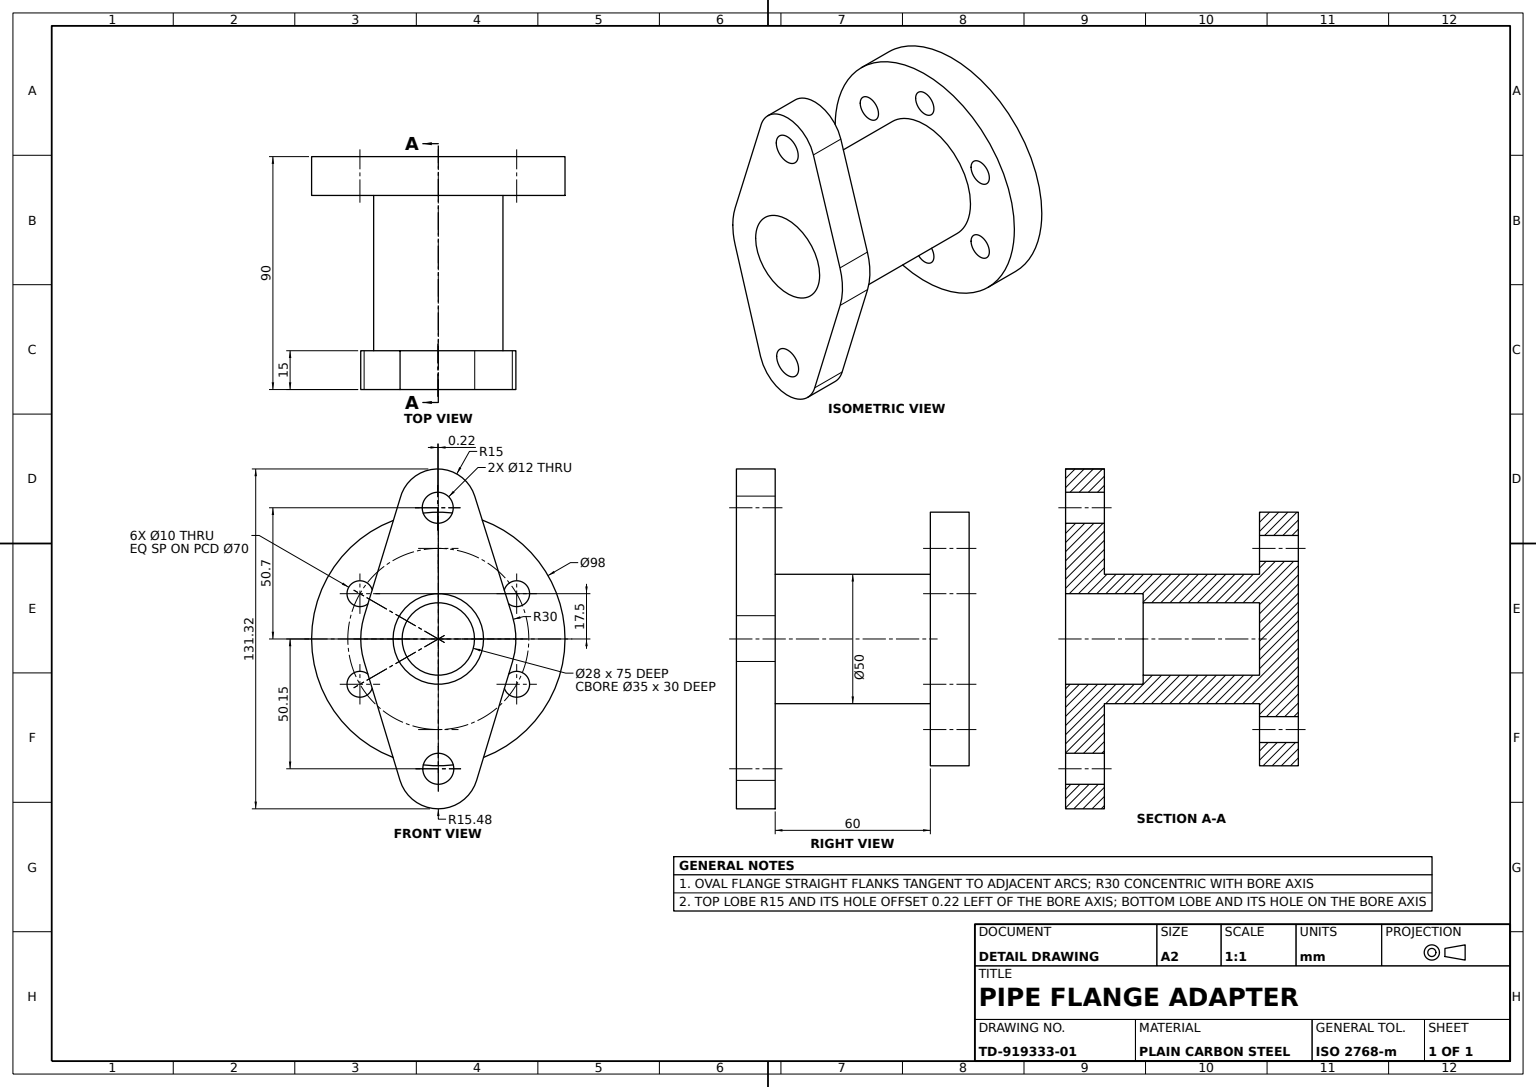
from build123d import *

# Parameters (mm, degrees)
ROUND_FLANGE_SKETCH_R          = 49
ROUND_FLANGE_98_DEPTH          = 15
ROUND_FLANGE_HOLES_SKETCH_R    = 5
ROUND_FLANGE_HOLES_6X_10_DEPTH = 15
SLEEVE_SKETCH_R                = 25
SLEEVE_50_DEPTH                = 60
OVAL_FLANGE_DEPTH              = 15
OVAL_FLANGE_HOLES_SKETCH_R     = 6
OVAL_FLANGE_HOLES_2X_12_DEPTH  = 15
COUNTERBORE_SKETCH_R           = 17.5
COUNTERBORE_35_DEPTH           = 30
BORE_SKETCH_R                  = 14
BORE_28_DEPTH                  = 45


with BuildPart() as part:
    # Round Flange Sketch → Round Flange Ø98 (new body)
    with BuildSketch(Plane.XY):
        Circle(ROUND_FLANGE_SKETCH_R)
    extrude(amount=ROUND_FLANGE_98_DEPTH)

    # Round Flange Holes Sketch → Round Flange Holes 6xØ10 (cut)
    with BuildSketch(Plane.XY.offset(15)):
        with Locations((0, 35)):
            Circle(ROUND_FLANGE_HOLES_SKETCH_R)
        with Locations((30.310889132, 17.5)):
            Circle(ROUND_FLANGE_HOLES_SKETCH_R)
        with Locations((30.310889132, -17.5)):
            Circle(ROUND_FLANGE_HOLES_SKETCH_R)
        with Locations((0, -35)):
            Circle(ROUND_FLANGE_HOLES_SKETCH_R)
        with Locations((-30.310889132, -17.5)):
            Circle(ROUND_FLANGE_HOLES_SKETCH_R)
        with Locations((-30.310889132, 17.5)):
            Circle(ROUND_FLANGE_HOLES_SKETCH_R)
    extrude(amount=-ROUND_FLANGE_HOLES_6X_10_DEPTH, mode=Mode.SUBTRACT)

    # Sleeve Sketch → Sleeve Ø50 (add)
    with BuildSketch(Plane.XY.offset(15)):
        Circle(SLEEVE_SKETCH_R)
    extrude(amount=SLEEVE_50_DEPTH)

    # Oval Flange Sketch → Oval Flange (add)
    with BuildSketch(Plane.XY.offset(75)):
        with BuildLine():
            Line((-14.812486777, -54.633777367), (-28.714375061, -8.688191115))
            ThreePointArc((-28.714375061, -8.688191115), (-29.999971167, 0.041592963), (-28.690173521, 8.7677787))
            Line((-28.690173521, 8.7677787), (-14.786489776, 54.263806016))
            ThreePointArc((-14.786489776, 54.263806016), (-0.706868372, 65.68836713), (14.083896835, 55.200774455))
            Line((14.083896835, 55.200774455), (28.617323634, 9.002710037))
            ThreePointArc((28.617323634, 9.002710037), (29.999548575, 0.16457607), (28.714375061, -8.688191115))
            Line((28.714375061, -8.688191115), (14.812486777, -54.633777367))
            ThreePointArc((14.812486777, -54.633777367), (0, -65.627604906), (-14.812486777, -54.633777367))
        make_face()
    extrude(amount=OVAL_FLANGE_DEPTH)

    # Oval Flange Holes Sketch → Oval Flange Holes 2xØ12 (cut)
    with BuildSketch(Plane.XY.offset(90)):
        with Locations((-0.220456426, 50.700774863)):
            Circle(OVAL_FLANGE_HOLES_SKETCH_R)
        with Locations((0, -50.151920606)):
            Circle(OVAL_FLANGE_HOLES_SKETCH_R)
    extrude(amount=-OVAL_FLANGE_HOLES_2X_12_DEPTH, mode=Mode.SUBTRACT)

    # Counterbore Sketch → Counterbore Ø35 (cut)
    with BuildSketch(Plane.XY.offset(90)):
        Circle(COUNTERBORE_SKETCH_R)
    extrude(amount=-COUNTERBORE_35_DEPTH, mode=Mode.SUBTRACT)

    # Bore Sketch → Bore Ø28 (cut)
    with BuildSketch(Plane.XY.offset(60)):
        Circle(BORE_SKETCH_R)
    extrude(amount=-BORE_28_DEPTH, mode=Mode.SUBTRACT)


solid = part.part
